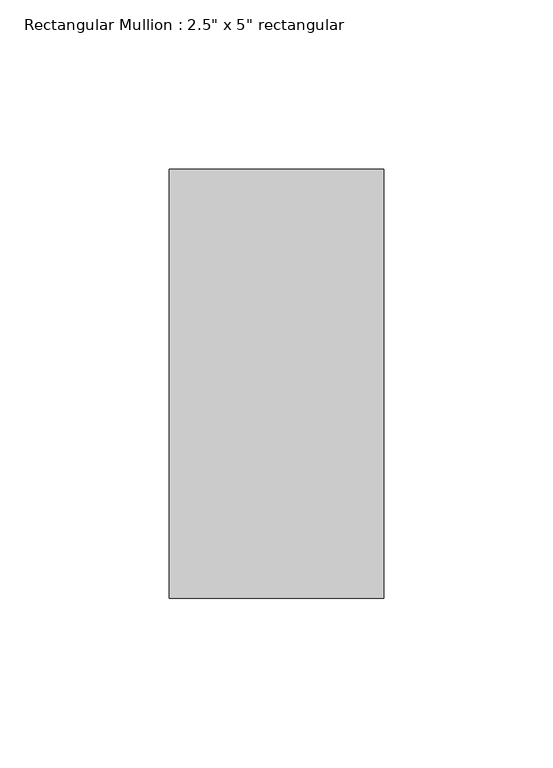
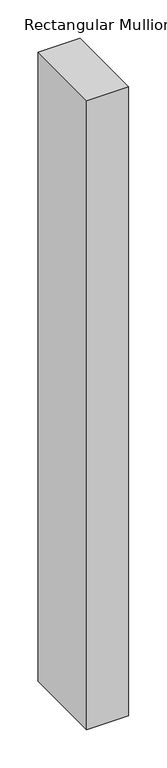
"""IFC4 building model written with IfcOpenShell, lengths in millimetres: member geometry."""

from ifc_helpers import new_model, si_unit, frame, origin, place, context, project, spatial, polyline, outline, extrude, source, transform, mapped, element, save


def member_b9dc02b9(model_context):
    return source(origin(), model_context, "Body", "SweptSolid", [
        extrude(outline(polyline([(31.75, 63.5), (31.75, -63.5), (-31.75, -63.5), (-31.75, 63.5), (31.75, 63.5)])), frame((0.0, 0.0, -1003.2999998), z_axis=(0.0, 0.0, 1.0), x_axis=(1.0, 0.0, 0.0)), (0.0, 0.0, 1.0), 1003.2999998),
    ])


if __name__ == "__main__":
    model = new_model("IFC4")
    model_context = context("Model", 3, world=origin())
    ifc_project = project(units=[si_unit("LENGTHUNIT", "METRE", prefix="MILLI")], contexts=[model_context])
    site = spatial("IfcSite", under=ifc_project)
    building = spatial("IfcBuilding", under=site)
    placement = place(None, origin())
    member_shape = member_b9dc02b9(model_context)
    element("IfcMember", 1, ObjectType="Rectangular Mullion : 2.5\" x 5\" rectangular", at=placement, inside=building, context=model_context, shape_type="MappedRepresentation", body=[
        mapped(member_shape, transform((0.0, 0.0, 0.0), x_axis=(1.0, 0.0, 0.0), y_axis=(0.0, 1.0, 0.0), z_axis=(0.0, 0.0, 1.0))),
    ])
    save(model, "model.ifc")

# Revit data of these elements
# Type "Rectangular Mullion : 2.5\" x 5\" rectangular"
#   built-in parameter 1007304 = 0.416667 (stored number, unit not read)
#   built-in parameter 1007301 = 0.104167 (stored number, unit not read)
#   built-in parameter 1007300 = 0.104167 (stored number, unit not read)
# Element 1 (IfcMember, "Rectangular Mullion : 2.5\" x 5\" rectangular")
#   Materials on its faces: "Aluminum"
# Materials
#   "Aluminum": class "Metal", colour RGB 247 247 247, transparency 0, Description = "Aluminum 6061", Cost = 0
